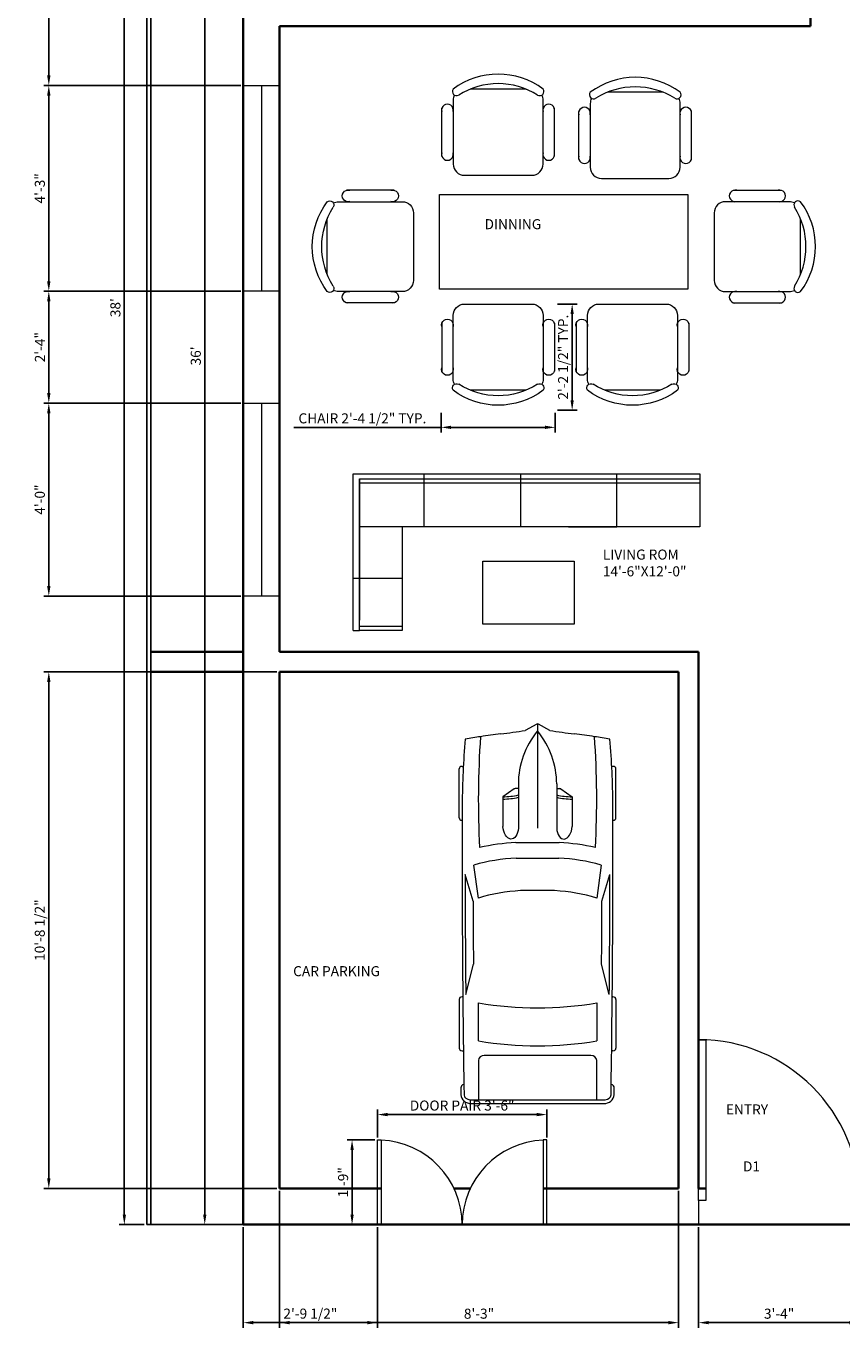
# Model space of a CAD drawing. Units: inches. Extents: x 0 to 3634, y 1847 to 2359.
# Tile 1 of 3: x 3218 to 3421, y 1847 to 2171. Entities that reach past the tile are written whole.
import ezdxf

# ---------------------------------------------------------------- set-up
doc = ezdxf.new("R2010")
doc.units = ezdxf.units.IN
for name, color, linetype, lineweight, true_color in [('A-ANNO-DIMS', 215, 'Continuous', 18, 0xa953a0), ('A-ANNO-TEXT', 215, 'Continuous', 18, 0xa953a0), ('A-AREA-IDEN', 9, 'Continuous', 18, 0xafd9aa), ('A-FURN', 254, 'Continuous', 18, 0xd7ebd2), ('A-GLAZ', 9, 'Continuous', 18, 0xafd9aa), ('C-PROP', 9, 'Continuous', 25, 0xafd9aa)]:
    doc.layers.add(name, color=color, linetype=linetype, lineweight=lineweight, true_color=true_color)
for name, color, linetype, lineweight in [('A-DOOR', 4, 'Continuous', 18), ('A-EQPM-VEHI', 8, 'Continuous', 13), ('A-WALL', 7, 'Continuous', 35)]:
    doc.layers.add(name, color=color, linetype=linetype, lineweight=lineweight)
doc.styles.get("Standard").update_dxf_attribs({"font": 'arial.ttf'})
doc.dimstyles.new('ISO-25', dxfattribs={"dimtxt": 2.5, "dimasz": 2.5, "dimexe": 1.25, "dimexo": 0.625, "dimtad": 1, "dimlunit": 3, "dimtxsty": 'Standard', "dimcen": 2.5, "dimadec": 0, "dimazin": 0, "dimtfac": 1, "dimtmove": 0, "dimatfit": 3, "dimfxl": 1, "dimarcsym": 0})

# ---------------------------------------------------------------- blocks, each defined once
blk = doc.blocks.new('CHAIR7')
for p, q in [((5.12, 15.04), (17.88, 15.04)), ((20, 12), (3, 12)), ((0, 9), (0, -9)), ((23, -7.44), (23, 7.44)), ((3, -12), (20, -12)), ((5.12, -15), (17.88, -15))]:
    blk.add_line(p, q)
for centre, radius, start, end in [((5.56, 13.54), 1.56, 73.7398, 286.2602), ((17.44, 13.54), 1.56, 253.7398, 106.2602), ((3, 9), 3, 90, 180), ((20, 9), 3, 62.4156, 90), ((22.34, 11.12), 1.1, 53.3099, 212.0274), ((4.82, 0), 19.64, 327.5758, 32.4242), ((7, 0), 20, 323.1301, 36.8699), ((3, -9), 3, 180, 270), ((5.56, -13.5), 1.56, 73.7398, 286.2602), ((17.44, -13.5), 1.56, 253.7398, 106.2602), ((20, -9), 3, 270, 297.5844), ((22.34, -11.12), 1.1, 147.9726, 306.6901)]:
    blk.add_arc(centre, radius, start, end)
blk = doc.blocks.new('*U3')
for p, q in [((46.55, 38.89), (22.35, 38.89)), ((136.7, 38.89), (160.9, 38.89)), ((21.1, 37.41), (21.1, 36.83)), ((47.8, 37.39), (47.8, 37.41)), ((87.99, 31.87), (74.76, 35.92)), ((134.31, 35.6), (119.29, 31.78)), ((135.45, 37.07), (135.45, 37.41)), ((162.15, 37.41), (162.15, 36.77)), ((186.47, -33.5), (186.47, 33.5)), ((188.4, -32.76), (188.4, 32.76)), ((70.03, 31.54), (86.41, 29.35)), ((138.42, 29.35), (157.25, 29.35)), ((164.52, 26.39), (164.52, -26.39)), ((186.47, 29.35), (167.01, 29.35)), ((32.27, 11.63), (36.13, 17.17)), ((36.13, 17.17), (50.94, 17.17)), ((29.77, 9.51), (51.68, 9.51)), ((32.12, 9.51), (32.12, 11.15)), ((58.92, -10.77), (58.92, 10.77)), ((66.55, -10.53), (66.55, 10.53)), ((82.74, 8.5), (82.74, -8.5)), ((186.47, -10.53), (186.47, 10.53)), ((3.27, 6.13), (0.1, 0.41)), ((0, 0), (51.68, 0)), ((0.1, -0.41), (3.27, -6.13)), ((29.77, -9.51), (51.68, -9.51)), ((32.12, -9.51), (32.12, -11.15)), ((32.27, -11.63), (36.13, -17.17)), ((36.13, -17.17), (50.94, -17.17)), ((86.41, -29.35), (70.03, -31.54)), ((87.99, -31.87), (74.76, -35.92)), ((134.31, -35.6), (119.29, -31.78)), ((157.25, -29.35), (138.42, -29.35)), ((167.01, -29.35), (186.47, -29.35)), ((21.1, -37.41), (21.1, -36.83)), ((47.8, -37.39), (47.8, -37.41)), ((135.45, -37.07), (135.45, -37.41)), ((162.15, -37.41), (162.15, -36.77)), ((46.55, -38.89), (22.35, -38.89)), ((136.7, -38.89), (160.9, -38.89))]:
    blk.add_line(p, q)
for centre, major_axis, ratio, start_param, end_param in [((22.35, 37.41), (0, -1.48), 0.842304, 3.141593, 4.712389), ((46.55, 37.41), (0, 1.48), 0.842304, -1.570796, 0), ((136.7, 37.41), (0, -1.48), 0.842304, 3.141593, 4.712389), ((160.9, 37.41), (0, 1.48), 0.842304, -1.570796, 0), ((266.03, -27.52), (0, 313.31), 0.842304, 1.367076, 1.39176), ((41.19, -490.86), (0, 528.23), 0.842304, 0.00281, 0.075598), ((64.48, -10555.62), (0, 10593.03), 0.842304, -0.013397, 0.002797), ((64.48, -10555.62), (0, -10591.55), 0.842304, 3.133765, 3.140441), ((180.63, 35.84), (0, 2.22), 0.842304, -0.013017, 1.249894), ((64.48, -10556.36), (0, 10595.31), 0.842304, -0.013397, -0.013017), ((183.98, 33.5), (0, -2.96), 0.842304, 1.570796, 3.128196), ((183.98, 32.76), (0, -5.25), 0.842304, 1.570796, 3.128196), ((259.18, -27.52), (0, -305.3), 0.842304, 4.528606, 4.561838), ((37.47, -593.96), (0, -623.33), 0.842304, 3.096046, 3.200911), ((134.4, 5.39), (0, -89.78), 0.842304, 4.449482, 4.652344), ((135.29, 5.39), (0, 81.77), 0.842304, 1.245306, 1.50788), ((149.6, 2.8), (0, -79.58), 0.842304, 4.372215, 4.640744), ((95.79, -3666.35), (0, -3698.24), 0.842304, 3.134049, 3.144098), ((17.08, 0), (0, 147.02), 0.842304, 4.511394, 4.913384), ((35.91, 0), (0, 147.02), 0.842304, 4.511394, 4.913384), ((167.01, 26.39), (0, 2.96), 0.842304, 0, 1.570796), ((-204.49, 52.4), (0, -250.96), 0.842304, 1.385369, 1.434372), ((13.04, 17.01), (0, 27.42), 0.842304, 4.435146, 4.718221), ((14.2, 17.01), (0, 27.42), 0.842304, 4.435146, 4.718221), ((50.79, 13.34), (6.34, -0.36), 0.603834, -1.395552, 1.581315), ((29.77, -46.66), (0, 56.17), 0.842304, 0, 0.590319), ((32.75, 11.15), (0, 0.74), 0.842304, 0.879714, 1.570796), ((0.62, 0), (0, -0.74), 0.842304, 4.131459, 5.293319), ((-204.49, -52.4), (0, 250.96), 0.842304, -1.434372, -1.385369), ((29.77, 46.66), (0, 56.17), 0.842304, 2.551274, 3.141593), ((32.75, -11.15), (0, -0.74), 0.842304, 4.712389, 5.403472), ((13.04, -17.01), (0, -27.42), 0.842304, 1.564964, 1.848039), ((14.2, -17.01), (0, -27.42), 0.842304, 1.564964, 1.848039), ((134.4, -5.39), (0, -89.78), 0.842304, -1.510751, -1.307889), ((135.29, -5.39), (0, -81.77), 0.842304, -1.50788, -1.245306), ((149.6, -2.8), (0, -79.58), 0.842304, -1.499151, -1.230623), ((259.18, 27.52), (0, 305.3), 0.842304, 1.721348, 1.754579), ((266.03, 27.52), (0, 313.31), 0.842304, 1.749832, 1.774517), ((37.47, 593.96), (0, -623.33), 0.842304, -0.059319, 0.045547), ((95.79, 3666.35), (0, -3698.24), 0.842304, -0.002505, 0.007544), ((167.01, -26.39), (0, -2.96), 0.842304, 4.712389, 6.283185), ((41.19, 490.86), (0, -528.23), 0.842304, -0.075598, -0.00281), ((22.35, -37.41), (0, 1.48), 0.842304, 1.570796, 3.141593), ((64.48, 10555.62), (0, 10593.03), 0.842304, 3.138796, 3.15499), ((46.55, -37.41), (0, -1.48), 0.842304, 0, 1.570796), ((64.48, 10555.62), (0, -10591.55), 0.842304, 0.001152, 0.007828), ((136.7, -37.41), (0, -1.48), 0.842304, -1.570796, 0), ((160.9, -37.41), (0, 1.48), 0.842304, 3.141593, 4.712389), ((180.63, -35.84), (0, -2.22), 0.842304, -1.249894, 0.013017), ((64.48, 10556.36), (0, 10595.31), 0.842304, 3.15461, 3.15499), ((183.98, -33.5), (0, 2.96), 0.842304, 3.15499, 4.712389), ((183.98, -32.76), (0, -5.25), 0.842304, 0.013397, 1.570796)]:
    blk.add_ellipse(centre, major_axis=major_axis, ratio=ratio, start_param=start_param, end_param=end_param)
at = {"extrusion": (0, 0, -1)}
blk.add_ellipse((50.79, -13.34), major_axis=(6.34, 0.36), ratio=0.603834, start_param=-1.395552, end_param=1.581315, dxfattribs=at)
blk = doc.blocks.new('*U7')
for p, q in [((0, 0), (0, -6)), ((40, 0), (40, -6))]:
    blk.add_line(p, q)
blk.add_lwpolyline([(0, 0), (0, 40), (1.75, 40), (1.75, 0)], close=True)
blk.add_arc((0, 0), 40, 0, 90)
blk = doc.blocks.new('DR-69P')
for points in [[(1.5, 0), (0, 0), (0, 34.5), (1.5, 34.5)], [(67.5, 0), (69, 0), (69, 34.5), (67.5, 34.5)]]:
    blk.add_lwpolyline(points, close=True)
for centre, start, end in [((0, 0), 0, 87.5104), ((69, 0), 92.4896, 180)]:
    blk.add_arc(centre, 34.5, start, end)
blk = doc.blocks.new('*D12')
at = {"layer": 'A-ANNO-DIMS', "color": 0, "lineweight": -2, "transparency": 16777216}
for p, q in [((3271.39, 2305.31), (3261.19, 2305.31)), ((3262.44, 2302.81), (3262.44, 1875.81)), ((3271.39, 1873.31), (3261.19, 1873.31))]:
    blk.add_line(p, q, dxfattribs=at)
at = {"layer": 'A-ANNO-DIMS', "color": 0, "transparency": 16777216}
for points in [[(3262.03, 2302.81), (3262.86, 2302.81), (3262.44, 2305.31)], [(3262.03, 1875.81), (3262.86, 1875.81), (3262.44, 1873.31)]]:
    blk.add_solid(points, dxfattribs=at)
at = {"layer": 'Defpoints', "color": 0, "transparency": 16777216}
for p in [(3272.02, 2305.31), (3262.44, 1873.31), (3272.02, 1873.31)]:
    blk.add_point(p, dxfattribs=at)
at = {"layer": 'A-ANNO-DIMS', "color": 0, "transparency": 16777216, "insert": (3260.54, 2089.31), "char_height": 2.5, "attachment_point": 5, "rotation": 90}
blk.add_mtext("36'", dxfattribs=at)
blk = doc.blocks.new('*D15')
at = {"layer": 'A-ANNO-DIMS', "color": 0, "lineweight": -2, "transparency": 16777216}
for p, q in [((3247.39, 2329.31), (3241.2, 2329.31)), ((3242.45, 1875.81), (3242.45, 2326.81)), ((3247.39, 1873.31), (3241.2, 1873.31))]:
    blk.add_line(p, q, dxfattribs=at)
at = {"layer": 'A-ANNO-DIMS', "color": 0, "transparency": 16777216}
for points in [[(3242.04, 2326.81), (3242.87, 2326.81), (3242.45, 2329.31)], [(3242.04, 1875.81), (3242.87, 1875.81), (3242.45, 1873.31)]]:
    blk.add_solid(points, dxfattribs=at)
at = {"layer": 'Defpoints', "color": 0, "transparency": 16777216}
for p in [(3242.45, 2329.31), (3248.02, 2329.31), (3248.02, 1873.31)]:
    blk.add_point(p, dxfattribs=at)
at = {"layer": 'A-ANNO-DIMS', "color": 0, "transparency": 16777216, "insert": (3240.55, 2101.31), "char_height": 2.5, "attachment_point": 5, "rotation": 90}
blk.add_mtext("38'", dxfattribs=at)
blk = doc.blocks.new('*D18')
at = {"layer": 'A-ANNO-DIMS', "color": 0, "lineweight": -2, "transparency": 16777216}
for p, q in [((3321.2, 2075.18), (3321.2, 2070.3)), ((3349.54, 2075.18), (3349.54, 2070.3)), ((3321.2, 2071.55), (3284.58, 2071.55)), ((3347.04, 2071.55), (3323.7, 2071.55))]:
    blk.add_line(p, q, dxfattribs=at)
at = {"layer": 'A-ANNO-DIMS', "color": 0, "transparency": 16777216}
for points in [[(3323.7, 2071.97), (3323.7, 2071.14), (3321.2, 2071.55)], [(3347.04, 2071.97), (3347.04, 2071.14), (3349.54, 2071.55)]]:
    blk.add_solid(points, dxfattribs=at)
at = {"layer": 'Defpoints', "color": 0, "transparency": 16777216}
for p in [(3321.2, 2075.8), (3349.54, 2075.8), (3321.2, 2071.55)]:
    blk.add_point(p, dxfattribs=at)
at = {"layer": 'A-ANNO-DIMS', "color": 0, "transparency": 16777216, "insert": (3301.64, 2073.47), "char_height": 2.5, "attachment_point": 5}
blk.add_mtext('CHAIR 2\'-4 1/2" TYP.', dxfattribs=at)
blk = doc.blocks.new('*D19')
at = {"layer": 'A-ANNO-DIMS', "color": 0, "lineweight": -2, "transparency": 16777216}
for p, q in [((3350.16, 2102.2), (3355.04, 2102.2)), ((3353.79, 2099.7), (3353.79, 2078.3)), ((3350.16, 2075.8), (3355.04, 2075.8))]:
    blk.add_line(p, q, dxfattribs=at)
at = {"layer": 'A-ANNO-DIMS', "color": 0, "transparency": 16777216}
for points in [[(3353.37, 2099.7), (3354.2, 2099.7), (3353.79, 2102.2)], [(3353.37, 2078.3), (3354.2, 2078.3), (3353.79, 2075.8)]]:
    blk.add_solid(points, dxfattribs=at)
at = {"layer": 'Defpoints', "color": 0, "transparency": 16777216}
for p in [(3349.54, 2102.2), (3349.54, 2075.8), (3353.79, 2075.8)]:
    blk.add_point(p, dxfattribs=at)
at = {"layer": 'A-ANNO-DIMS', "color": 0, "transparency": 16777216, "insert": (3351.87, 2089), "char_height": 2.5, "attachment_point": 5, "rotation": 90}
blk.add_mtext('2\'-2 1/2" TYP.', dxfattribs=at)
blk = doc.blocks.new('*D24')
at = {"layer": 'A-ANNO-DIMS', "color": 0, "lineweight": -2, "transparency": 16777216}
for p, q in [((3305.39, 1894.98), (3305.39, 1901.92)), ((3307.89, 1900.67), (3344.99, 1900.67)), ((3347.49, 1894.98), (3347.49, 1901.92))]:
    blk.add_line(p, q, dxfattribs=at)
at = {"layer": 'A-ANNO-DIMS', "color": 0, "transparency": 16777216}
for points in [[(3307.89, 1901.09), (3307.89, 1900.26), (3305.39, 1900.67)], [(3344.99, 1901.09), (3344.99, 1900.26), (3347.49, 1900.67)]]:
    blk.add_solid(points, dxfattribs=at)
at = {"layer": 'Defpoints', "color": 0, "transparency": 16777216}
for p in [(3347.49, 1900.67), (3305.39, 1894.36), (3347.49, 1894.36)]:
    blk.add_point(p, dxfattribs=at)
at = {"layer": 'A-ANNO-DIMS', "color": 0, "transparency": 16777216, "insert": (3326.44, 1902.59), "char_height": 2.5, "attachment_point": 5}
blk.add_mtext('DOOR PAIR 3\'-6"', dxfattribs=at)
blk = doc.blocks.new('*D25')
at = {"layer": 'A-ANNO-DIMS', "color": 0, "lineweight": -2, "transparency": 16777216}
for p, q in [((3304.76, 1894.36), (3297.82, 1894.36)), ((3299.07, 1875.81), (3299.07, 1891.86)), ((3304.76, 1873.31), (3297.82, 1873.31))]:
    blk.add_line(p, q, dxfattribs=at)
at = {"layer": 'A-ANNO-DIMS', "color": 0, "transparency": 16777216}
for points in [[(3298.66, 1891.86), (3299.49, 1891.86), (3299.07, 1894.36)], [(3298.66, 1875.81), (3299.49, 1875.81), (3299.07, 1873.31)]]:
    blk.add_solid(points, dxfattribs=at)
at = {"layer": 'Defpoints', "color": 0, "transparency": 16777216}
for p in [(3299.07, 1894.36), (3305.39, 1894.36), (3305.39, 1873.31)]:
    blk.add_point(p, dxfattribs=at)
at = {"layer": 'A-ANNO-DIMS', "color": 0, "transparency": 16777216, "insert": (3297.17, 1883.83), "char_height": 2.5, "attachment_point": 5, "rotation": 90}
blk.add_mtext('1\'-9"', dxfattribs=at)
blk = doc.blocks.new('*D26')
at = {"layer": 'A-ANNO-DIMS', "color": 0, "lineweight": -2, "transparency": 16777216}
for p, q in [((3281.02, 1881.68), (3281.02, 1847.68)), ((3380.24, 1881.68), (3380.24, 1847.68)), ((3283.52, 1848.93), (3377.74, 1848.93))]:
    blk.add_line(p, q, dxfattribs=at)
at = {"layer": 'A-ANNO-DIMS', "color": 0, "transparency": 16777216}
for points in [[(3283.52, 1849.35), (3283.52, 1848.52), (3281.02, 1848.93)], [(3377.74, 1849.35), (3377.74, 1848.52), (3380.24, 1848.93)]]:
    blk.add_solid(points, dxfattribs=at)
at = {"layer": 'Defpoints', "color": 0, "transparency": 16777216}
for p in [(3281.02, 1882.31), (3380.24, 1882.31), (3380.24, 1848.93)]:
    blk.add_point(p, dxfattribs=at)
at = {"layer": 'A-ANNO-DIMS', "color": 0, "transparency": 16777216, "insert": (3330.63, 1850.84), "char_height": 2.5, "attachment_point": 5}
blk.add_mtext('8\'-3"', dxfattribs=at)
blk = doc.blocks.new('*D27')
at = {"layer": 'A-ANNO-DIMS', "color": 0, "lineweight": -2, "transparency": 16777216}
for p, q in [((3280.39, 2010.76), (3222.42, 2010.76)), ((3223.67, 1884.81), (3223.67, 2008.26)), ((3280.39, 1882.31), (3222.42, 1882.31))]:
    blk.add_line(p, q, dxfattribs=at)
at = {"layer": 'A-ANNO-DIMS', "color": 0, "transparency": 16777216}
for points in [[(3223.25, 2008.26), (3224.09, 2008.26), (3223.67, 2010.76)], [(3223.25, 1884.81), (3224.09, 1884.81), (3223.67, 1882.31)]]:
    blk.add_solid(points, dxfattribs=at)
at = {"layer": 'Defpoints', "color": 0, "transparency": 16777216}
for p in [(3223.67, 2010.76), (3281.02, 2010.76), (3281.02, 1882.31)]:
    blk.add_point(p, dxfattribs=at)
at = {"layer": 'A-ANNO-DIMS', "color": 0, "transparency": 16777216, "insert": (3221.75, 1946.53), "char_height": 2.5, "attachment_point": 5, "rotation": 90}
blk.add_mtext('10\'-8 1/2"', dxfattribs=at)
blk = doc.blocks.new('*D28')
at = {"layer": 'A-ANNO-DIMS', "color": 0, "lineweight": -2, "transparency": 16777216}
for p, q in [((3385.24, 1872.66), (3385.24, 1847.68)), ((3425.24, 1872.66), (3425.24, 1847.68)), ((3387.74, 1848.93), (3422.74, 1848.93))]:
    blk.add_line(p, q, dxfattribs=at)
at = {"layer": 'A-ANNO-DIMS', "color": 0, "transparency": 16777216}
for points in [[(3387.74, 1849.35), (3387.74, 1848.52), (3385.24, 1848.93)], [(3422.74, 1849.35), (3422.74, 1848.52), (3425.24, 1848.93)]]:
    blk.add_solid(points, dxfattribs=at)
at = {"layer": 'Defpoints', "color": 0, "transparency": 16777216}
for p in [(3385.24, 1873.28), (3425.24, 1873.28), (3425.24, 1848.93)]:
    blk.add_point(p, dxfattribs=at)
at = {"layer": 'A-ANNO-DIMS', "color": 0, "transparency": 16777216, "insert": (3405.24, 1850.84), "char_height": 2.5, "attachment_point": 5}
blk.add_mtext('3\'-4"', dxfattribs=at)
blk = doc.blocks.new('*D34')
at = {"layer": 'A-ANNO-DIMS', "color": 0, "lineweight": -2, "transparency": 16777216}
for p, q in [((3271.39, 2077.57), (3222.42, 2077.57)), ((3223.67, 2032.1), (3223.67, 2075.07)), ((3271.39, 2029.6), (3222.42, 2029.6))]:
    blk.add_line(p, q, dxfattribs=at)
at = {"layer": 'A-ANNO-DIMS', "color": 0, "transparency": 16777216}
for points in [[(3223.25, 2075.07), (3224.09, 2075.07), (3223.67, 2077.57)], [(3223.25, 2032.1), (3224.09, 2032.1), (3223.67, 2029.6)]]:
    blk.add_solid(points, dxfattribs=at)
at = {"layer": 'Defpoints', "color": 0, "transparency": 16777216}
for p in [(3223.67, 2077.57), (3272.02, 2077.57), (3272.02, 2029.6)]:
    blk.add_point(p, dxfattribs=at)
at = {"layer": 'A-ANNO-DIMS', "color": 0, "transparency": 16777216, "insert": (3221.77, 2053.59), "char_height": 2.5, "attachment_point": 5, "rotation": 90}
blk.add_mtext('4\'-0"', dxfattribs=at)
blk = doc.blocks.new('*D35')
at = {"layer": 'A-ANNO-DIMS', "color": 0, "lineweight": -2, "transparency": 16777216}
for p, q in [((3271.39, 2105.4), (3222.42, 2105.4)), ((3223.67, 2080.07), (3223.67, 2102.9)), ((3271.39, 2077.57), (3222.42, 2077.57))]:
    blk.add_line(p, q, dxfattribs=at)
at = {"layer": 'A-ANNO-DIMS', "color": 0, "transparency": 16777216}
for points in [[(3223.25, 2102.9), (3224.09, 2102.9), (3223.67, 2105.4)], [(3223.25, 2080.07), (3224.09, 2080.07), (3223.67, 2077.57)]]:
    blk.add_solid(points, dxfattribs=at)
at = {"layer": 'Defpoints', "color": 0, "transparency": 16777216}
for p in [(3223.67, 2105.4), (3272.02, 2105.4), (3272.02, 2077.57)]:
    blk.add_point(p, dxfattribs=at)
at = {"layer": 'A-ANNO-DIMS', "color": 0, "transparency": 16777216, "insert": (3221.79, 2091.49), "char_height": 2.5, "attachment_point": 5, "rotation": 90}
blk.add_mtext('2\'-4"', dxfattribs=at)
blk = doc.blocks.new('*D36')
at = {"layer": 'A-ANNO-DIMS', "color": 0, "lineweight": -2, "transparency": 16777216}
for p, q in [((3271.39, 2156.56), (3222.42, 2156.56)), ((3223.67, 2107.9), (3223.67, 2154.06)), ((3271.39, 2105.4), (3222.42, 2105.4))]:
    blk.add_line(p, q, dxfattribs=at)
at = {"layer": 'A-ANNO-DIMS', "color": 0, "transparency": 16777216}
for points in [[(3223.25, 2154.06), (3224.09, 2154.06), (3223.67, 2156.56)], [(3223.25, 2107.9), (3224.09, 2107.9), (3223.67, 2105.4)]]:
    blk.add_solid(points, dxfattribs=at)
at = {"layer": 'Defpoints', "color": 0, "transparency": 16777216}
for p in [(3223.67, 2156.56), (3272.02, 2156.56), (3272.02, 2105.4)]:
    blk.add_point(p, dxfattribs=at)
at = {"layer": 'A-ANNO-DIMS', "color": 0, "transparency": 16777216, "insert": (3221.77, 2130.98), "char_height": 2.5, "attachment_point": 5, "rotation": 90}
blk.add_mtext('4\'-3"', dxfattribs=at)
blk = doc.blocks.new('*D37')
at = {"layer": 'A-ANNO-DIMS', "color": 0, "lineweight": -2, "transparency": 16777216}
for p, q in [((3271.39, 2305.31), (3222.42, 2305.31)), ((3223.67, 2159.06), (3223.67, 2302.81)), ((3271.39, 2156.56), (3222.42, 2156.56))]:
    blk.add_line(p, q, dxfattribs=at)
at = {"layer": 'A-ANNO-DIMS', "color": 0, "transparency": 16777216}
for points in [[(3223.25, 2302.81), (3224.09, 2302.81), (3223.67, 2305.31)], [(3223.25, 2159.06), (3224.09, 2159.06), (3223.67, 2156.56)]]:
    blk.add_solid(points, dxfattribs=at)
at = {"layer": 'Defpoints', "color": 0, "transparency": 16777216}
for p in [(3223.67, 2305.31), (3272.02, 2305.31), (3272.02, 2156.56)]:
    blk.add_point(p, dxfattribs=at)
at = {"layer": 'A-ANNO-DIMS', "color": 0, "transparency": 16777216, "insert": (3221.75, 2230.93), "char_height": 2.5, "attachment_point": 5, "rotation": 90}
blk.add_mtext('12\'-4 1/2"', dxfattribs=at)
blk = doc.blocks.new('*D44')
at = {"layer": 'A-ANNO-DIMS', "color": 0, "lineweight": -2, "transparency": 16777216}
for p, q in [((3272.02, 1872.68), (3272.02, 1847.68)), ((3305.39, 1872.68), (3305.39, 1847.68)), ((3274.52, 1848.93), (3302.89, 1848.93))]:
    blk.add_line(p, q, dxfattribs=at)
at = {"layer": 'A-ANNO-DIMS', "color": 0, "transparency": 16777216}
for points in [[(3274.52, 1849.35), (3274.52, 1848.52), (3272.02, 1848.93)], [(3302.89, 1849.35), (3302.89, 1848.52), (3305.39, 1848.93)]]:
    blk.add_solid(points, dxfattribs=at)
at = {"layer": 'Defpoints', "color": 0, "transparency": 16777216}
for p in [(3272.02, 1873.31), (3305.39, 1873.31), (3305.39, 1848.93)]:
    blk.add_point(p, dxfattribs=at)
at = {"layer": 'A-ANNO-DIMS', "color": 0, "transparency": 16777216, "insert": (3288.7, 1850.85), "char_height": 2.5, "attachment_point": 5}
blk.add_mtext('2\'-9 1/2"', dxfattribs=at)

msp = doc.modelspace()

# ---------------------------------------------------------------- linework, layer by layer
at = {"layer": 'A-FURN'}
for p, q in [((3299.323, 2060.02), (3385.515, 2060.02)), ((3299.323, 2021.063), (3299.323, 2060.02)), ((3300.923, 2058.793), (3300.923, 2023.647)), ((3300.923, 2021.063), (3300.923, 2058.793)), ((3300.923, 2058.793), (3385.515, 2058.793)), ((3316.92, 2060.02), (3316.92, 2046.793)), ((3316.92, 2060.02), (3328.92, 2060.02)), ((3328.92, 2060.02), (3340.92, 2060.02)), ((3340.92, 2060.02), (3340.92, 2046.793)), ((3340.92, 2060.02), (3352.92, 2060.02)), ((3364.92, 2046.793), (3364.92, 2060.02)), ((3385.515, 2060.02), (3385.515, 2058.793)), ((3385.515, 2058.793), (3385.515, 2046.793)), ((3300.923, 2057.793), (3385.515, 2057.793)), ((3311.529, 2046.793), (3300.923, 2046.793)), ((3385.515, 2046.793), (3311.529, 2046.793)), ((3311.529, 2046.793), (3311.529, 2021.063)), ((3352.92, 2046.793), (3364.92, 2046.793)), ((3311.529, 2033.928), (3299.323, 2033.928)), ((3299.323, 2021.063), (3300.923, 2021.063)), ((3311.529, 2022.063), (3300.923, 2022.063)), ((3311.529, 2021.063), (3300.923, 2021.063))]:
    msp.add_line(p, q, dxfattribs=at)
for points in [[(3320.805, 2129.477), (3382.588, 2129.477), (3382.588, 2105.934), (3320.805, 2105.934)], [(3331.596, 2038.248), (3354.264, 2038.248), (3354.264, 2022.612), (3331.596, 2022.612)]]:
    msp.add_lwpolyline(points, close=True, dxfattribs=at)
at = {"layer": 'A-GLAZ'}
for p, q in [((3272.018, 2156.56), (3281.018, 2156.56)), ((3272.018, 2105.401), (3272.018, 2156.56)), ((3272.018, 2156.56), (3276.518, 2156.56)), ((3276.518, 2156.56), (3276.518, 2105.401)), ((3281.018, 2156.56), (3281.018, 2105.401)), ((3281.018, 2105.401), (3272.018, 2105.401)), ((3272.018, 2077.57), (3281.018, 2077.57)), ((3272.018, 2029.604), (3272.018, 2077.57)), ((3272.018, 2077.57), (3276.518, 2077.57)), ((3276.518, 2077.57), (3276.518, 2029.604)), ((3281.018, 2077.57), (3281.018, 2029.604)), ((3281.018, 2029.604), (3272.018, 2029.604))]:
    msp.add_line(p, q, dxfattribs=at)
at = {"layer": 'A-WALL'}
for p, q in [((3272.018, 1873.309), (3272.018, 2305.309)), ((3413.018, 2171.309), (3413.018, 2213.309)), ((3281.018, 2171.309), (3413.018, 2171.309)), ((3281.018, 2053.307), (3281.018, 2171.309)), ((3281.018, 2015.759), (3281.018, 2053.307)), ((3272.018, 2015.759), (3249.018, 2015.759)), ((3281.018, 2015.759), (3385.237, 2015.759)), ((3385.237, 2015.759), (3385.237, 1882.309)), ((3272.018, 2010.759), (3249.018, 2010.759)), ((3281.018, 1882.309), (3281.018, 2010.759)), ((3281.018, 2010.759), (3380.237, 2010.759)), ((3380.237, 2010.759), (3380.237, 1882.309)), ((3306.304, 1882.309), (3281.018, 1882.309)), ((3328.46, 1882.309), (3324.418, 1882.309)), ((3380.237, 1882.309), (3346.573, 1882.309)), ((3386.987, 1882.309), (3385.237, 1882.309)), ((3584.018, 1873.309), (3272.018, 1873.309))]:
    msp.add_line(p, q, dxfattribs=at)
at = {"layer": 'C-PROP'}
for p, q in [((3248.018, 2329.309), (3248.018, 1873.309)), ((3249.018, 2329.309), (3249.018, 1873.309)), ((3248.018, 1873.309), (3272.018, 1873.309))]:
    msp.add_line(p, q, dxfattribs=at)

# ---------------------------------------------------------------- block references
at = {"layer": 'A-DOOR'}
msp.add_blockref('*U7', (3385.237, 1879.283), dxfattribs=at)
at = {"layer": 'A-DOOR', "xscale": 0.6101383878996555, "yscale": 0.6101383878996555, "zscale": 0.6101383878996555}
msp.add_blockref('DR-69P', (3305.389, 1873.309), dxfattribs=at)
at = {"layer": 'A-EQPM-VEHI', "xscale": 0.501173325400758, "yscale": 0.501173325400758, "zscale": 0.501173325400758, "rotation": 270}
msp.add_blockref('*U3', (3345.177, 1997.82), dxfattribs=at)
at = {"layer": 'A-FURN', "yscale": 0.9316886440311337, "zscale": 0.9316886440311337, "rotation": 90}
for p, xscale in [((3335.389, 2134.235), 0.9316886440311337), ((3369.469, 2133.434), 0.9316886440311337), ((3335.389, 2102.202), -0.9316886440311337), ((3368.79, 2102.202), -0.9316886440311337)]:
    msp.add_blockref('CHAIR7', p, dxfattribs=dict(at, xscale=xscale))
at = {"layer": 'A-FURN', "yscale": 0.9316886440311337, "zscale": 0.9316886440311337}
for p, xscale in [((3314.335, 2116.484), -0.9316886440311337), ((3389.134, 2116.484), 0.9316886440311337)]:
    msp.add_blockref('CHAIR7', p, dxfattribs=dict(at, xscale=xscale))

# ---------------------------------------------------------------- texts
at = {"layer": 'A-ANNO-TEXT', "insert": (3396.26, 1889.035), "char_height": 2.5, "attachment_point": 1}
msp.add_mtext_dynamic_manual_height_columns('D1', width=11.51191, gutter_width=12.5, heights=[0], dxfattribs=at)
at = {"layer": 'A-AREA-IDEN', "char_height": 2.5, "attachment_point": 1}
for s, width, insert in [('DINNING', 37.24106, (3332.01, 2123.322)), ('LIVING ROM\\P14\'-6"X12\'-0"', 32.81614, (3361.407, 2041.169)), ('CAR PARKING', 31.43718, (3284.42, 1937.578)), ('ENTRY', 16.38539, (3392.008, 1903.197))]:
    msp.add_mtext_dynamic_manual_height_columns(s, width=width, gutter_width=12.5, heights=[0], dxfattribs=dict(at, insert=insert))

# ---------------------------------------------------------------- dimensions: what is measured, and where the dimension line sits
at = {"layer": 'A-ANNO-DIMS'}
for base, p1, p2, override, picture, middle in [((3242.454, 2329.309), (3248.018, 1873.309), (3248.018, 2329.309), {"dimclrd": 0, "dimclre": 0, "dimclrt": 0}, '*D15', (3240.552, 2101.309)), ((3223.668, 2305.309), (3272.018, 2156.56), (3272.018, 2305.309), {"dimdec": 1, "dimlfac": 1, "dimrnd": 0, "dimzin": 1, "dimdsep": 46, "dimlunit": 4, "dimfrac": 2}, '*D37', (3221.751, 2230.934)), ((3262.442, 1873.309), (3272.018, 2305.309), (3272.018, 1873.309), {"dimclrd": 0, "dimclre": 0, "dimclrt": 0}, '*D12', (3260.54, 2089.309)), ((3223.668, 2156.56), (3272.018, 2105.401), (3272.018, 2156.56), {"dimdec": 1, "dimlfac": 1, "dimrnd": 0, "dimzin": 1, "dimdsep": 46, "dimlunit": 4, "dimfrac": 2}, '*D36', (3221.766, 2130.98)), ((3223.668, 2105.401), (3272.018, 2077.57), (3272.018, 2105.401), {"dimdec": 1, "dimlfac": 1, "dimrnd": 0, "dimzin": 1, "dimdsep": 46, "dimlunit": 4, "dimfrac": 2}, '*D35', (3221.788, 2091.486)), ((3223.668, 2077.57), (3272.018, 2029.604), (3272.018, 2077.57), {"dimdec": 1, "dimlfac": 1, "dimrnd": 0, "dimzin": 1, "dimdsep": 46, "dimlunit": 4, "dimfrac": 2}, '*D34', (3221.767, 2053.587)), ((3223.6683, 2010.7591), (3281.0183, 1882.3089), (3281.0183, 2010.7591), {"dimdec": 1, "dimlfac": 1, "dimrnd": 0, "dimzin": 1, "dimdsep": 46, "dimlunit": 4, "dimfrac": 2}, '*D27', (3221.7507, 1946.534)), ((3299.0739, 1894.3587), (3305.3888, 1873.3089), (3305.3888, 1894.3587), {"dimdec": 1, "dimlfac": 1, "dimrnd": 0, "dimzin": 1, "dimdsep": 46, "dimlunit": 4, "dimfrac": 2}, '*D25', (3297.1724, 1883.8338))]:
    dim = msp.add_linear_dim(base=base, p1=p1, p2=p2, angle=90, dimstyle='ISO-25', override=override, dxfattribs=at)
    dim.commit()
    dim.dimension.update_dxf_attribs({"geometry": picture, "text_midpoint": middle})
for base, p1, p2, angle, text, picture, middle in [((3353.788, 2075.804), (3349.538, 2102.202), (3349.538, 2075.804), 270, '<> TYP.', '*D19', (3351.871, 2089.003)), ((3321.201, 2071.554), (3349.538, 2075.804), (3321.201, 2075.804), 180, 'CHAIR <> TYP.', '*D18', (3301.64, 2073.471))]:
    dim = msp.add_linear_dim(base=base, p1=p1, p2=p2, angle=angle, text=text, dimstyle='ISO-25', override={"dimdec": 1, "dimlfac": 1, "dimrnd": 0, "dimzin": 1, "dimdsep": 46, "dimlunit": 4, "dimfrac": 2}, dxfattribs=at)
    dim.commit()
    dim.dimension.update_dxf_attribs({"geometry": picture, "text_midpoint": middle})
dim = msp.add_linear_dim(base=(3347.488, 1900.674), p1=(3305.389, 1894.359), p2=(3347.488, 1894.359), text='DOOR PAIR <>', dimstyle='ISO-25', override={"dimdec": 1, "dimlfac": 1, "dimrnd": 0, "dimzin": 1, "dimdsep": 46, "dimlunit": 4, "dimfrac": 2}, dxfattribs=at)
dim.commit()
dim.dimension.update_dxf_attribs({"geometry": '*D24', "text_midpoint": (3326.439, 1902.593)})
for base, p1, p2, picture, middle in [((3380.237, 1848.933), (3281.018, 1882.309), (3380.237, 1882.309), '*D26', (3330.628, 1850.836)), ((3305.389, 1848.933), (3272.018, 1873.309), (3305.389, 1873.309), '*D44', (3288.704, 1850.851)), ((3425.237, 1848.933), (3385.237, 1873.283), (3425.237, 1873.283), '*D28', (3405.237, 1850.836))]:
    dim = msp.add_linear_dim(base=base, p1=p1, p2=p2, dimstyle='ISO-25', override={"dimdec": 1, "dimlfac": 1, "dimrnd": 0, "dimzin": 1, "dimdsep": 46, "dimlunit": 4, "dimfrac": 2}, dxfattribs=at)
    dim.commit()
    dim.dimension.update_dxf_attribs({"geometry": picture, "text_midpoint": middle})

doc.saveas('drawing.dxf')
